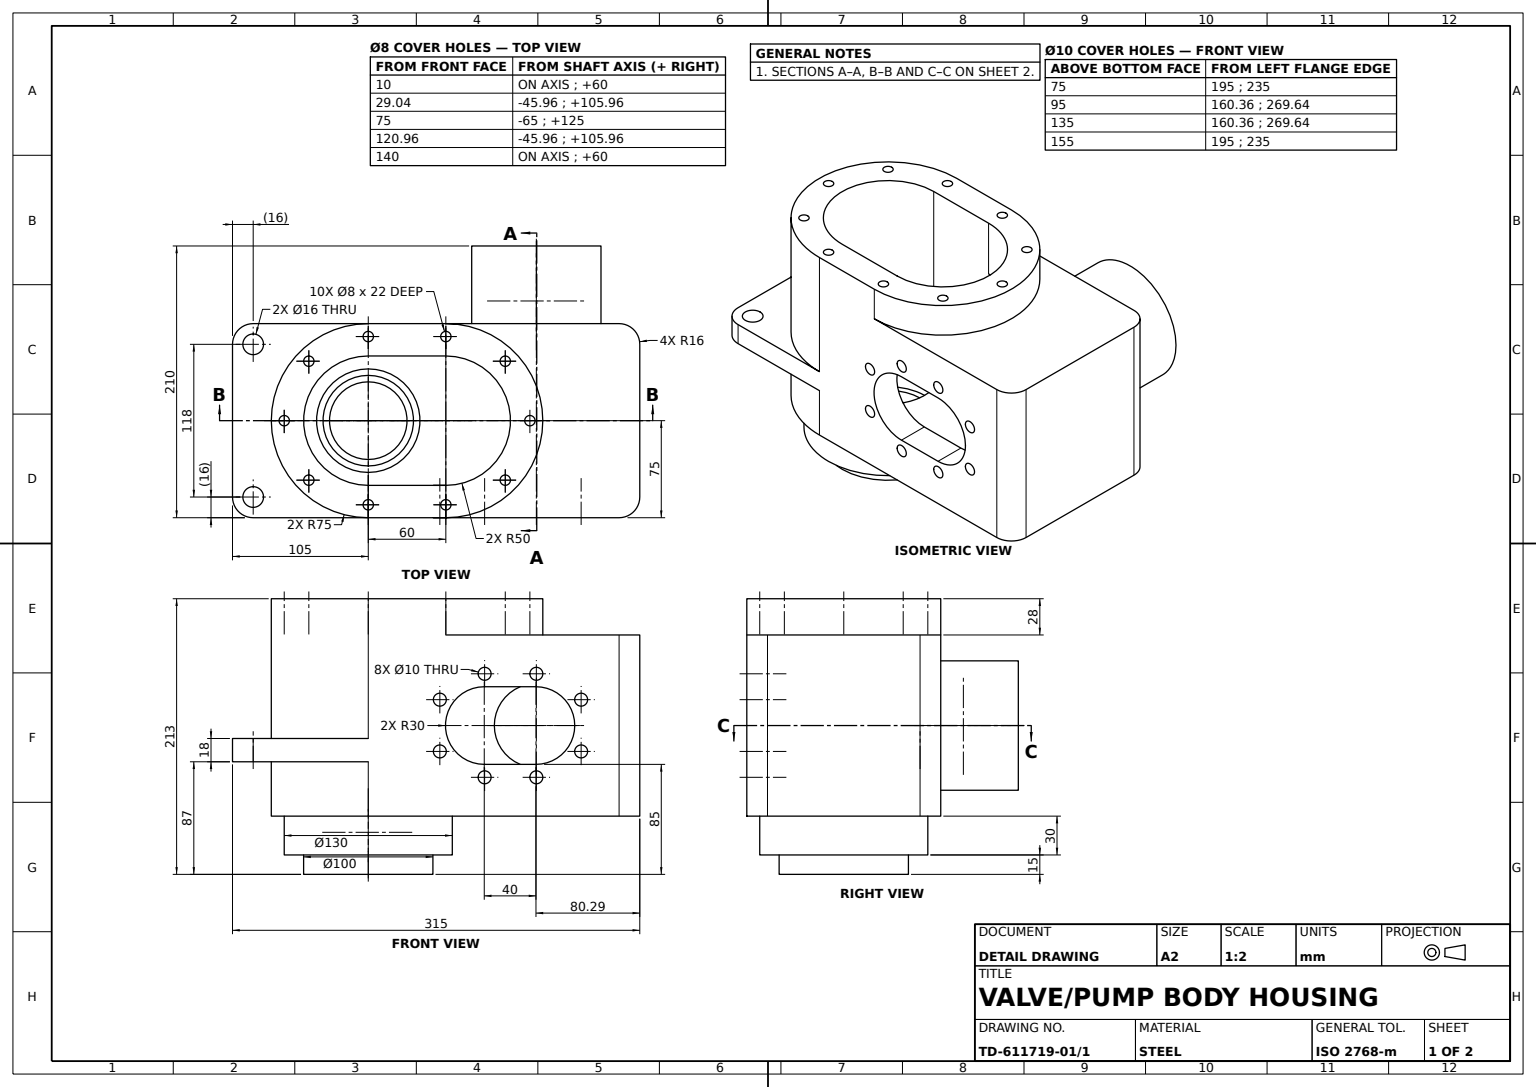
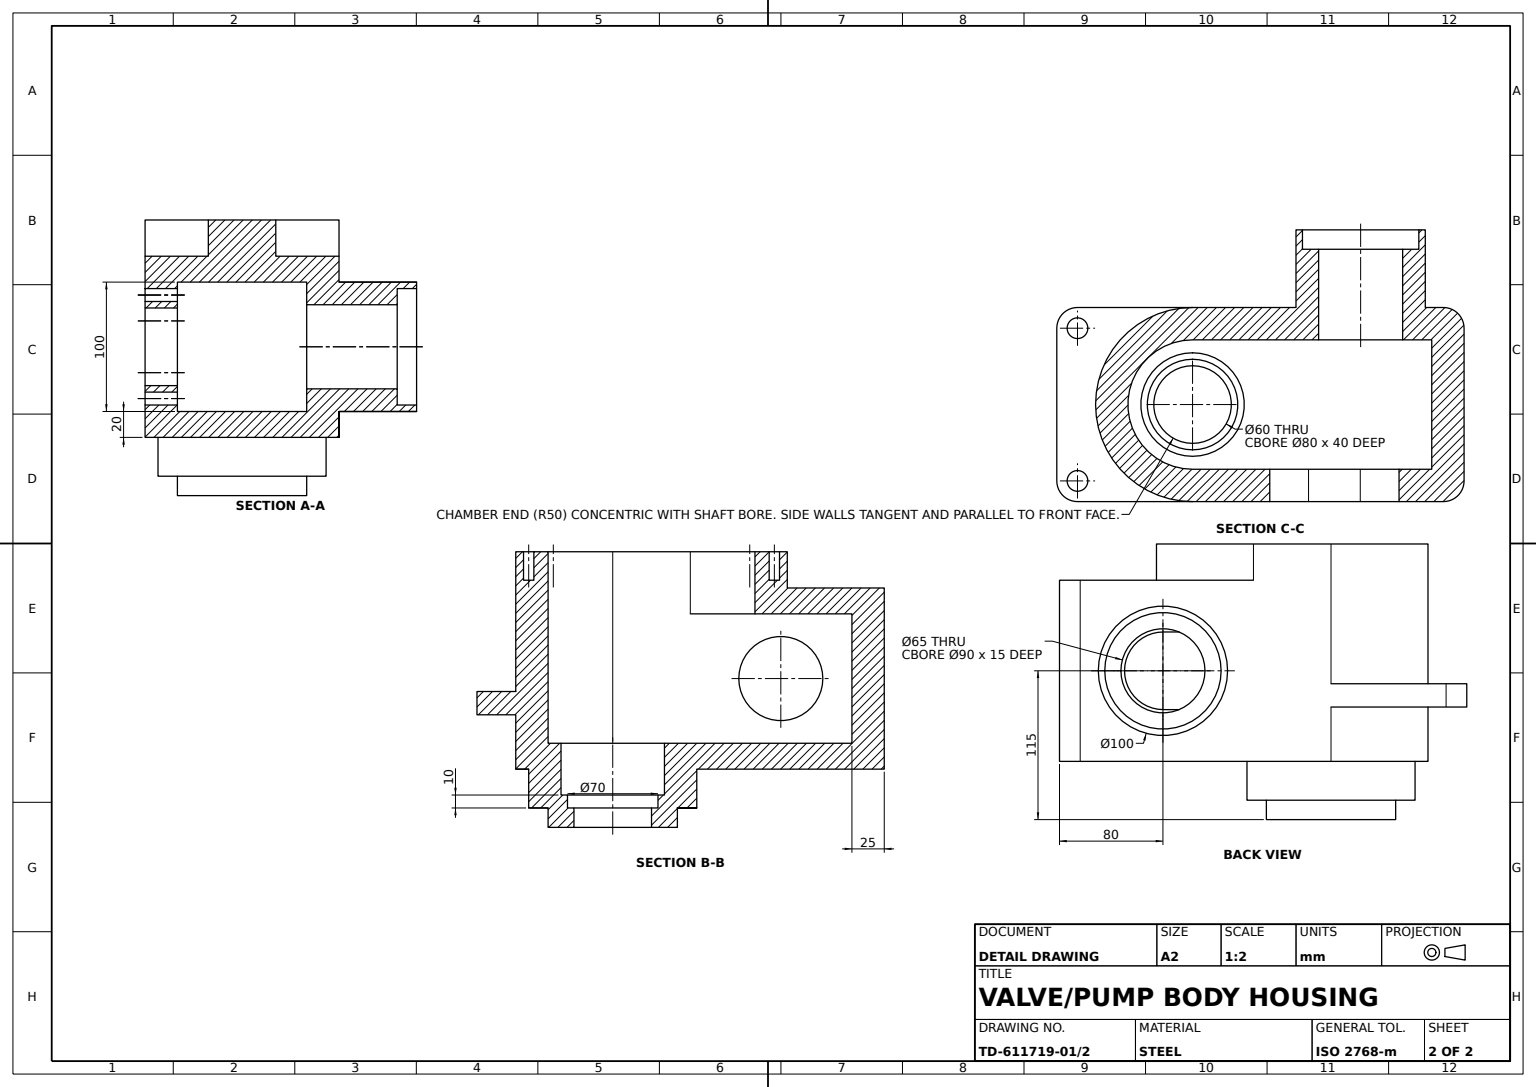
from build123d import *

# Parameters (mm, degrees)
BASE_BOSS_SKETCH_R         = 50
BASE_BOSS_100_DEPTH        = 15
BEARING_BOSS_SKETCH_R      = 65
BEARING_BOSS_130_DEPTH     = 30
HOUSING_BLOCK_75X210_DEPTH = 168
HOUSING_RECESS_CUT_DEPTH   = 28
MOUNTING_FLANGE_DEPTH      = 18
GEAR_CAVITY_SKETCH_R       = 5
GEAR_CAVITY_CUT_DEPTH      = 94
CAVITY_RELIEF_CUT_DEPTH    = 94
PORT_BOSS_SKETCH_R         = 50
PORT_BOSS_100_DEPTH        = 60
PORT_COUNTERBORE_SKETCH_R  = 45
PORT_COUNTERBORE_90_DEPTH  = 15
PORT_BORE_SKETCH_R         = 32.5
PORT_BORE_65_DEPTH         = 150
SIDE_POCKET_50X185_DEPTH   = 50
BASE_BORE_SKETCH_R         = 30
BASE_BORE_60_DEPTH         = 15
BASE_COUNTERBORE_SKETCH_R  = 35
BASE_COUNTERBORE_70_DEPTH  = 10
SHAFT_BORE_SKETCH_R        = 40
SHAFT_BORE_80_DEPTH        = 119
COVER_BOLT_HOLES_SKETCH_R  = 4
COVER_BOLT_HOLES_8_DEPTH   = 22
FLANGE_FILLET_R16_A_R      = 16
FLANGE_FILLET_R16_B_R      = 16
FLANGE_BOLT_HOLES_SKETCH_R = 8
FLANGE_BOLT_HOLES_16_DEPTH = 91
INNER_START                = -91
INNER_SLOT_CUT_DEPTH       = 91
HOUSING_FILLET_R16_A_R     = 16
HOUSING_FILLET_R16_B_R     = 16


with BuildPart() as part:
    # Base Boss Sketch → Base Boss Ø100 (new body)
    with BuildSketch(Plane(origin=(0, 0, 0), x_dir=(1, 0, 0), z_dir=(0, 1, 0))):
        with Locations(Location((0, 0, 0), (0, 0, 270))):
            Circle(BASE_BOSS_SKETCH_R)
    extrude(amount=BASE_BOSS_100_DEPTH)

    # Bearing Boss Sketch → Bearing Boss Ø130 (add)
    with BuildSketch(Plane(origin=(0, 15, 0), x_dir=(1, 0, 0), z_dir=(0, 1, 0))):
        with Locations(Location((0, 0, 0), (0, 0, 270))):
            Circle(BEARING_BOSS_SKETCH_R)
    extrude(amount=BEARING_BOSS_130_DEPTH)

    # Housing Block Sketch → Housing Block 75x210 (add)
    with BuildSketch(Plane(origin=(0, 45, 0), x_dir=(1, 0, 0), z_dir=(0, 1, 0))):
        with BuildLine():
            Line((0, -75), (210, -75))
            Line((210, -75), (210, 75))
            Line((210, 75), (0, 75))
            ThreePointArc((0, 75), (-75, 0), (0, -75))
        make_face()
    extrude(amount=HOUSING_BLOCK_75X210_DEPTH)

    # Housing Recess Sketch → Housing Recess Cut (cut)
    with BuildSketch(Plane(origin=(0, 213, 0), x_dir=(1, 0, 0), z_dir=(0, 1, 0))):
        with BuildLine():
            Line((60, 75), (210, 75))
            Line((210, 75), (210, -75))
            Line((210, -75), (60, -75))
            ThreePointArc((60, -75), (135, 0), (60, 75))
        make_face()
    extrude(amount=-HOUSING_RECESS_CUT_DEPTH, mode=Mode.SUBTRACT)

    # Mounting Flange Sketch → Mounting Flange (add)
    with BuildSketch(Plane(origin=(0, 87, 0), x_dir=(-1, 0, 0), z_dir=(0, -1, 0))):
        with BuildLine():
            Line((105, 0), (105, 75))
            Line((105, 75), (0, 75))
            ThreePointArc((0, 75), (75, 0), (0, -75))
            Line((0, -75), (105, -75))
            Line((105, -75), (105, 0))
        make_face()
    extrude(amount=-MOUNTING_FLANGE_DEPTH)

    # Gear Cavity Sketch → Gear Cavity Cut (cut)
    with BuildSketch(Plane.XY.offset(75)):
        with Locations((130, 155)):
            Circle(GEAR_CAVITY_SKETCH_R)
        with Locations((90, 155)):
            Circle(GEAR_CAVITY_SKETCH_R)
        with Locations((164.641016151, 135)):
            Circle(GEAR_CAVITY_SKETCH_R)
        with Locations((164.641016151, 95)):
            Circle(GEAR_CAVITY_SKETCH_R)
        with Locations((130, 75)):
            Circle(GEAR_CAVITY_SKETCH_R)
        with Locations((90, 75)):
            Circle(GEAR_CAVITY_SKETCH_R)
        with Locations((55.358983849, 95)):
            Circle(GEAR_CAVITY_SKETCH_R)
        with Locations((55.358983849, 135)):
            Circle(GEAR_CAVITY_SKETCH_R)
    extrude(amount=-GEAR_CAVITY_CUT_DEPTH, mode=Mode.SUBTRACT)

    # Cavity Relief Sketch → Cavity Relief Cut (cut)
    with BuildSketch(Plane.XY.offset(75)):
        with BuildLine():
            Line((89.708684664, 145), (129.708684664, 145))
            ThreePointArc((129.708684664, 145), (159.708684664, 115), (129.708684664, 85))
            Line((129.708684664, 85), (89.708684664, 85))
            ThreePointArc((89.708684664, 85), (59.708684664, 115), (89.708684664, 145))
        make_face()
    extrude(amount=-CAVITY_RELIEF_CUT_DEPTH, mode=Mode.SUBTRACT)

    # Port Boss Sketch → Port Boss Ø100 (add)
    with BuildSketch(Plane(origin=(0, 0, -75), x_dir=(-1, 0, 0), z_dir=(0, 0, -1))):
        with Locations(Location((-130, 115, 0), (0, 0, 180))):
            Circle(PORT_BOSS_SKETCH_R)
    extrude(amount=PORT_BOSS_100_DEPTH)

    # Port Counterbore Sketch → Port Counterbore Ø90 (cut)
    with BuildSketch(Plane(origin=(0, 0, -135), x_dir=(-1, 0, 0), z_dir=(0, 0, -1))):
        with Locations((-130, 115)):
            Circle(PORT_COUNTERBORE_SKETCH_R)
    extrude(amount=-PORT_COUNTERBORE_90_DEPTH, mode=Mode.SUBTRACT)

    # Port Bore Sketch → Port Bore Ø65 (cut)
    with BuildSketch(Plane(origin=(0, 0, -120), x_dir=(-1, 0, 0), z_dir=(0, 0, -1))):
        with Locations((-130, 115)):
            Circle(PORT_BORE_SKETCH_R)
    extrude(amount=-PORT_BORE_65_DEPTH, mode=Mode.SUBTRACT)

    # Side Pocket Sketch → Side Pocket 50x185 (cut, symmetric)
    with BuildSketch(Plane(origin=(0, 115, 0), x_dir=(-1, 0, 0), z_dir=(0, -1, 0))):
        with BuildLine():
            Line((0, 50), (-185, 50))
            Line((-185, 50), (-185, -50))
            Line((-185, -50), (0, -50))
            ThreePointArc((0, -50), (50, 0), (0, 50))
        make_face()
    extrude(amount=SIDE_POCKET_50X185_DEPTH, both=True, mode=Mode.SUBTRACT)

    # Base Bore Sketch → Base Bore Ø60 (cut)
    with BuildSketch(Plane.XZ):
        with Locations(Location((0, 0, 0), (0, 0, 270))):
            Circle(BASE_BORE_SKETCH_R)
    extrude(amount=-BASE_BORE_60_DEPTH, mode=Mode.SUBTRACT)

    # Base Counterbore Sketch → Base Counterbore Ø70 (cut)
    with BuildSketch(Plane.XZ.offset(-15)):
        with Locations(Location((0, 0, 0), (0, 0, 270))):
            Circle(BASE_COUNTERBORE_SKETCH_R)
    extrude(amount=-BASE_COUNTERBORE_70_DEPTH, mode=Mode.SUBTRACT)

    # Shaft Bore Sketch → Shaft Bore Ø80 (cut)
    with BuildSketch(Plane.XZ.offset(-25)):
        with Locations(Location((0, 0, 0), (0, 0, 270))):
            Circle(SHAFT_BORE_SKETCH_R)
    extrude(amount=-SHAFT_BORE_80_DEPTH, mode=Mode.SUBTRACT)

    # Cover Bolt Holes Sketch → Cover Bolt Holes Ø8 (cut)
    with BuildSketch(Plane(origin=(0, 213, 0), x_dir=(1, 0, 0), z_dir=(0, 1, 0))):
        with Locations(Location((125, 0, 0), (0, 0, 270))):
            Circle(COVER_BOLT_HOLES_SKETCH_R)
        with Locations(Location((105.961940777, 45.961940777, 0), (0, 0, 270))):
            Circle(COVER_BOLT_HOLES_SKETCH_R)
        with Locations(Location((105.961940777, -45.961940777, 0), (0, 0, 270))):
            Circle(COVER_BOLT_HOLES_SKETCH_R)
        with Locations(Location((60, -65, 0), (0, 0, 270))):
            Circle(COVER_BOLT_HOLES_SKETCH_R)
        with Locations(Location((0, -65, 0), (0, 0, 270))):
            Circle(COVER_BOLT_HOLES_SKETCH_R)
        with Locations(Location((-45.961940777, -45.961940777, 0), (0, 0, 270))):
            Circle(COVER_BOLT_HOLES_SKETCH_R)
        with Locations(Location((-45.961940777, 45.961940777, 0), (0, 0, 270))):
            Circle(COVER_BOLT_HOLES_SKETCH_R)
        with Locations(Location((0, 65, 0), (0, 0, 270))):
            Circle(COVER_BOLT_HOLES_SKETCH_R)
        with Locations(Location((60, 65, 0), (0, 0, 270))):
            Circle(COVER_BOLT_HOLES_SKETCH_R)
        with Locations(Location((-65, 0, 0), (0, 0, 270))):
            Circle(COVER_BOLT_HOLES_SKETCH_R)
    extrude(amount=-COVER_BOLT_HOLES_8_DEPTH, mode=Mode.SUBTRACT)

    # Flange Fillet R16 A
    flange_fillet_r16_a_edges = [part.edges().sort_by_distance(p)[0] for p in [
        (-105, 96, 75),
    ]]
    fillet(flange_fillet_r16_a_edges, radius=FLANGE_FILLET_R16_A_R)

    # Flange Fillet R16 B
    flange_fillet_r16_b_edges = [part.edges().sort_by_distance(p)[0] for p in [
        (-105, 96, -75),
    ]]
    fillet(flange_fillet_r16_b_edges, radius=FLANGE_FILLET_R16_B_R)

    # Flange Bolt Holes Sketch → Flange Bolt Holes Ø16 (cut)
    with BuildSketch(Plane(origin=(0, 105, 0), x_dir=(1, 0, 0), z_dir=(0, 1, 0))):
        with Locations(Location((-89, 59, 0), (0, 0, 270))):
            Circle(FLANGE_BOLT_HOLES_SKETCH_R)
        with Locations(Location((-89, -59, 0), (0, 0, 270))):
            Circle(FLANGE_BOLT_HOLES_SKETCH_R)
    extrude(amount=-FLANGE_BOLT_HOLES_16_DEPTH, mode=Mode.SUBTRACT)

    # Inner Slot Sketch → Inner Slot Cut (cut)
    with BuildSketch(Plane(origin=(0, 213, 0), x_dir=(1, 0, 0), z_dir=(0, 1, 0)).offset(INNER_START)):
        with BuildLine():
            Line((60, -50), (0, -50))
            ThreePointArc((0, -50), (-50, 0), (0, 50))
            Line((0, 50), (60, 50))
            ThreePointArc((60, 50), (110, 0), (60, -50))
        make_face()
    extrude(amount=INNER_SLOT_CUT_DEPTH, mode=Mode.SUBTRACT)

    # Housing Fillet R16 A
    housing_fillet_r16_a_edges = [part.edges().sort_by_distance(p)[0] for p in [
        (210, 115, -75),
    ]]
    fillet(housing_fillet_r16_a_edges, radius=HOUSING_FILLET_R16_A_R)

    # Housing Fillet R16 B
    housing_fillet_r16_b_edges = [part.edges().sort_by_distance(p)[0] for p in [
        (210, 115, 75),
    ]]
    fillet(housing_fillet_r16_b_edges, radius=HOUSING_FILLET_R16_B_R)


solid = part.part
